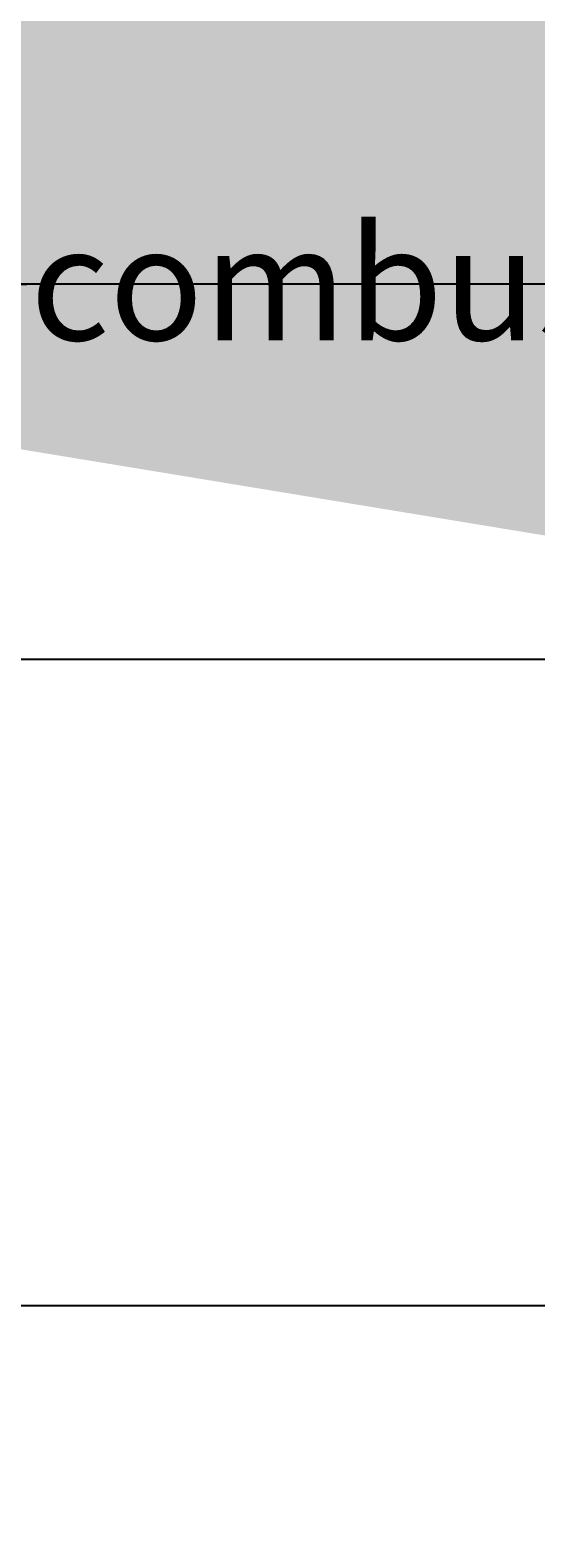
# Model space of a CAD drawing. Units: millimetres. Extents: x -22994 to 29398, y -19990 to 20176.
# Tile 53 of 135: x 216 to 229, y 25 to 65. Entities that reach past the tile are written whole.
import ezdxf
from ezdxf import colors
from ezdxf.entities.mleader import LeaderData, LeaderLine
from ezdxf.math import Vec2, Vec3

# ---------------------------------------------------------------- set-up
doc = ezdxf.new("R2010")
doc.units = ezdxf.units.MM
doc.header["$MEASUREMENT"] = 0
doc.layers.add('M-ANNO-TEXT', color=7, linetype='Continuous', lineweight=25)
doc.layers.add('M-DIMS', color=2, linetype='Continuous', lineweight=18)
doc.styles.get("Standard").update_dxf_attribs({"font": 'arial.ttf'})
doc.dimstyles.get("Standard").update_dxf_attribs({"dimtxt": 0.18, "dimasz": 10000, "dimexe": 0.18, "dimexo": 0.0625, "dimgap": 0.09, "dimtad": 0, "dimtih": 1, "dimtoh": 1, "dimdec": 0, "dimzin": 0, "dimdsep": 46, "dimtxsty": 'Standard', "dimcen": 0.09, "dimadec": 0, "dimazin": 0, "dimtfac": 1, "dimtdec": 0, "dimtofl": 0, "dimtmove": 0, "dimatfit": 3, "dimfxl": 1, "dimtolj": 1, "dimtzin": 0, "dimlwd": 30, "dimarcsym": 0})

# ---------------------------------------------------------------- blocks, each defined once
blk = doc.blocks.new('*D2')
at = {"layer": 'Defpoints', "color": 0, "transparency": 16777216}
for p in [(6.677, 10.271), (290.852, 10.271), (290.852, -5.079)]:
    blk.add_point(p, dxfattribs=at)
at = {"layer": 'M-DIMS', "color": 0, "lineweight": -2, "transparency": 16777216}
for p, q in [((6.677, 10.209), (6.677, -5.259)), ((290.852, 10.209), (290.852, -5.259))]:
    blk.add_line(p, q, dxfattribs=at)
at = {"layer": 'M-DIMS', "color": 0, "lineweight": 30, "transparency": 16777216}
for p, q in [((-9993.323, -5.079), (-19993.323, -5.079)), ((10290.852, -5.079), (20290.852, -5.079))]:
    blk.add_line(p, q, dxfattribs=at)
at = {"layer": 'M-DIMS', "color": 0, "transparency": 16777216}
for points in [[(-9993.323, 1661.588), (-9993.323, -1671.745), (6.677, -5.079)], [(10290.852, 1661.588), (10290.852, -1671.745), (290.852, -5.079)]]:
    blk.add_solid(points, dxfattribs=at)
at = {"layer": 'M-DIMS', "color": 0, "transparency": 16777216, "insert": (148.765, -5.079), "char_height": 0.18, "attachment_point": 5}
blk.add_mtext('\\A1;284.2', dxfattribs=at)
blk = doc.blocks.new('*D3')
at = {"layer": 'Defpoints', "color": 0, "transparency": 16777216}
for p in [(110.265, 204.165), (110.265, 176.366), (95.833, 127.967)]:
    blk.add_point(p, dxfattribs=at)
at = {"layer": 'M-DIMS', "color": 0, "lineweight": -2, "transparency": 16777216}
for p, q in [((95.833, 128.03), (95.833, 204.345)), ((110.265, 176.429), (110.265, 204.345))]:
    blk.add_line(p, q, dxfattribs=at)
at = {"layer": 'M-DIMS', "color": 0, "lineweight": 30, "transparency": 16777216}
for p, q in [((-9904.167, 204.165), (-19904.167, 204.165)), ((10110.265, 204.165), (20110.265, 204.165))]:
    blk.add_line(p, q, dxfattribs=at)
at = {"layer": 'M-DIMS', "color": 0, "transparency": 16777216}
for points in [[(-9904.167, 1870.832), (-9904.167, -1462.501), (95.833, 204.165)], [(10110.265, 1870.832), (10110.265, -1462.501), (110.265, 204.165)]]:
    blk.add_solid(points, dxfattribs=at)
at = {"layer": 'M-DIMS', "color": 0, "transparency": 16777216, "insert": (103.049, 204.165), "char_height": 0.18, "attachment_point": 5}
blk.add_mtext('\\A1;14.432', dxfattribs=at)
blk = doc.blocks.new('*D4')
at = {"layer": 'Defpoints', "color": 0, "transparency": 16777216}
for p in [(116.265, 204.165), (110.265, 176.366), (116.265, 176.366)]:
    blk.add_point(p, dxfattribs=at)
at = {"layer": 'M-DIMS', "color": 0, "lineweight": -2, "transparency": 16777216}
for p, q in [((110.265, 176.429), (110.265, 204.345)), ((116.265, 176.429), (116.265, 204.345))]:
    blk.add_line(p, q, dxfattribs=at)
at = {"layer": 'M-DIMS', "color": 0, "lineweight": 30, "transparency": 16777216}
for p, q in [((-9889.735, 204.165), (-19889.735, 204.165)), ((10116.265, 204.165), (20116.265, 204.165))]:
    blk.add_line(p, q, dxfattribs=at)
at = {"layer": 'M-DIMS', "color": 0, "transparency": 16777216}
for points in [[(-9889.735, 1870.832), (-9889.735, -1462.501), (110.265, 204.165)], [(10116.265, 1870.832), (10116.265, -1462.501), (116.265, 204.165)]]:
    blk.add_solid(points, dxfattribs=at)
at = {"layer": 'M-DIMS', "color": 0, "transparency": 16777216, "insert": (113.265, 204.165), "char_height": 0.18, "attachment_point": 5}
blk.add_mtext('\\A1;6', dxfattribs=at)
blk = doc.blocks.new('*D5')
at = {"layer": 'Defpoints', "color": 0, "transparency": 16777216}
for p in [(181.265, 204.165), (116.265, 176.366), (181.265, 176.366)]:
    blk.add_point(p, dxfattribs=at)
at = {"layer": 'M-DIMS', "color": 0, "lineweight": -2, "transparency": 16777216}
for p, q in [((116.265, 176.429), (116.265, 204.345)), ((181.265, 176.429), (181.265, 204.345))]:
    blk.add_line(p, q, dxfattribs=at)
at = {"layer": 'M-DIMS', "color": 0, "lineweight": 30, "transparency": 16777216}
for p, q in [((-9883.735, 204.165), (-19883.735, 204.165)), ((10181.265, 204.165), (20181.265, 204.165))]:
    blk.add_line(p, q, dxfattribs=at)
at = {"layer": 'M-DIMS', "color": 0, "transparency": 16777216}
for points in [[(-9883.735, 1870.832), (-9883.735, -1462.501), (116.265, 204.165)], [(10181.265, 1870.832), (10181.265, -1462.501), (181.265, 204.165)]]:
    blk.add_solid(points, dxfattribs=at)
at = {"layer": 'M-DIMS', "color": 0, "transparency": 16777216, "insert": (148.765, 204.165), "char_height": 0.18, "attachment_point": 5}
blk.add_mtext('\\A1;65', dxfattribs=at)
blk = doc.blocks.new('*D6')
at = {"layer": 'Defpoints', "color": 0, "transparency": 16777216}
for p in [(187.265, 204.165), (181.265, 176.366), (187.265, 176.366)]:
    blk.add_point(p, dxfattribs=at)
at = {"layer": 'M-DIMS', "color": 0, "lineweight": -2, "transparency": 16777216}
for p, q in [((181.265, 176.429), (181.265, 204.345)), ((187.265, 176.429), (187.265, 204.345))]:
    blk.add_line(p, q, dxfattribs=at)
at = {"layer": 'M-DIMS', "color": 0, "lineweight": 30, "transparency": 16777216}
for p, q in [((-9818.735, 204.165), (-19818.735, 204.165)), ((10187.265, 204.165), (20187.265, 204.165))]:
    blk.add_line(p, q, dxfattribs=at)
at = {"layer": 'M-DIMS', "color": 0, "transparency": 16777216}
for points in [[(-9818.735, 1870.832), (-9818.735, -1462.501), (181.265, 204.165)], [(10187.265, 1870.832), (10187.265, -1462.501), (187.265, 204.165)]]:
    blk.add_solid(points, dxfattribs=at)
at = {"layer": 'M-DIMS', "color": 0, "transparency": 16777216, "insert": (184.265, 204.165), "char_height": 0.18, "attachment_point": 5}
blk.add_mtext('\\A1;6', dxfattribs=at)
blk = doc.blocks.new('*D7')
at = {"layer": 'Defpoints', "color": 0, "transparency": 16777216}
for p in [(201.697, 204.165), (187.265, 176.366), (201.697, 127.967)]:
    blk.add_point(p, dxfattribs=at)
at = {"layer": 'M-DIMS', "color": 0, "lineweight": -2, "transparency": 16777216}
for p, q in [((187.265, 176.429), (187.265, 204.345)), ((201.697, 128.03), (201.697, 204.345))]:
    blk.add_line(p, q, dxfattribs=at)
at = {"layer": 'M-DIMS', "color": 0, "lineweight": 30, "transparency": 16777216}
for p, q in [((-9812.735, 204.165), (-19812.735, 204.165)), ((10201.697, 204.165), (20201.697, 204.165))]:
    blk.add_line(p, q, dxfattribs=at)
at = {"layer": 'M-DIMS', "color": 0, "transparency": 16777216}
for points in [[(-9812.735, 1870.832), (-9812.735, -1462.501), (187.265, 204.165)], [(10201.697, 1870.832), (10201.697, -1462.501), (201.697, 204.165)]]:
    blk.add_solid(points, dxfattribs=at)
at = {"layer": 'M-DIMS', "color": 0, "transparency": 16777216, "insert": (194.481, 204.165), "char_height": 0.18, "attachment_point": 5}
blk.add_mtext('\\A1;14.432', dxfattribs=at)
blk = doc.blocks.new('*D8')
at = {"layer": 'Defpoints', "color": 0, "transparency": 16777216}
for p in [(227.648, 204.165), (227.648, 146.73), (201.697, 127.967)]:
    blk.add_point(p, dxfattribs=at)
at = {"layer": 'M-DIMS', "color": 0, "lineweight": -2, "transparency": 16777216}
for p, q in [((201.697, 128.03), (201.697, 204.345)), ((227.648, 146.792), (227.648, 204.345))]:
    blk.add_line(p, q, dxfattribs=at)
at = {"layer": 'M-DIMS', "color": 0, "lineweight": 30, "transparency": 16777216}
for p, q in [((-9798.303, 204.165), (-19798.303, 204.165)), ((10227.648, 204.165), (20227.648, 204.165))]:
    blk.add_line(p, q, dxfattribs=at)
at = {"layer": 'M-DIMS', "color": 0, "transparency": 16777216}
for points in [[(-9798.303, 1870.832), (-9798.303, -1462.501), (201.697, 204.165)], [(10227.648, 1870.832), (10227.648, -1462.501), (227.648, 204.165)]]:
    blk.add_solid(points, dxfattribs=at)
at = {"layer": 'M-DIMS', "color": 0, "transparency": 16777216, "insert": (214.673, 204.165), "char_height": 0.18, "attachment_point": 5}
blk.add_mtext('\\A1;25.95', dxfattribs=at)
blk = doc.blocks.new('*D9')
at = {"layer": 'Defpoints', "color": 0, "transparency": 16777216}
for p in [(187.265, 176.366), (306.202, 176.366), (290.852, 10.271)]:
    blk.add_point(p, dxfattribs=at)
at = {"layer": 'M-DIMS', "color": 0, "lineweight": 30, "transparency": 16777216}
for p, q in [((306.202, 10176.366), (306.202, 20176.366)), ((306.202, -9989.729), (306.202, -19989.729))]:
    blk.add_line(p, q, dxfattribs=at)
at = {"layer": 'M-DIMS', "color": 0, "lineweight": -2, "transparency": 16777216}
for p, q in [((187.327, 176.366), (306.382, 176.366)), ((290.915, 10.271), (306.382, 10.271))]:
    blk.add_line(p, q, dxfattribs=at)
at = {"layer": 'M-DIMS', "color": 0, "transparency": 16777216}
for points in [[(-1360.465, 10176.366), (1972.869, 10176.366), (306.202, 176.366)], [(-1360.465, -9989.729), (1972.869, -9989.729), (306.202, 10.271)]]:
    blk.add_solid(points, dxfattribs=at)
at = {"layer": 'M-DIMS', "color": 0, "transparency": 16777216, "insert": (306.202, 93.319), "char_height": 0.18, "attachment_point": 5}
blk.add_mtext('\\A1;166.1', dxfattribs=at)
blk = doc.blocks.new('*D10')
at = {"layer": 'Defpoints', "color": 0, "transparency": 16777216}
for p in [(125.65, 136.071), (133.346, 136.071), (133.346, -5.079)]:
    blk.add_point(p, dxfattribs=at)
at = {"layer": 'M-DIMS', "color": 0, "lineweight": -2, "transparency": 16777216}
for p, q in [((125.65, 136.009), (125.65, -5.259)), ((133.346, 136.009), (133.346, -5.259))]:
    blk.add_line(p, q, dxfattribs=at)
at = {"layer": 'M-DIMS', "color": 0, "lineweight": 30, "transparency": 16777216}
for p, q in [((-9874.35, -5.079), (-19874.35, -5.079)), ((10133.346, -5.079), (20133.346, -5.079))]:
    blk.add_line(p, q, dxfattribs=at)
at = {"layer": 'M-DIMS', "color": 0, "transparency": 16777216}
for points in [[(-9874.35, 1661.588), (-9874.35, -1671.745), (125.65, -5.079)], [(10133.346, 1661.588), (10133.346, -1671.745), (133.346, -5.079)]]:
    blk.add_solid(points, dxfattribs=at)
at = {"layer": 'M-DIMS', "color": 0, "transparency": 16777216, "insert": (129.498, -5.079), "char_height": 0.18, "attachment_point": 5}
blk.add_mtext('\\A1;7.696', dxfattribs=at)
blk = doc.blocks.new('*D11')
at = {"layer": 'Defpoints', "color": 0, "transparency": 16777216}
for p in [(133.346, 136.071), (135.65, 136.071), (135.65, -5.079)]:
    blk.add_point(p, dxfattribs=at)
at = {"layer": 'M-DIMS', "color": 0, "lineweight": -2, "transparency": 16777216}
for p, q in [((133.346, 136.009), (133.346, -5.259)), ((135.65, 136.009), (135.65, -5.259))]:
    blk.add_line(p, q, dxfattribs=at)
at = {"layer": 'M-DIMS', "color": 0, "lineweight": 30, "transparency": 16777216}
for p, q in [((-9866.654, -5.079), (-19866.654, -5.079)), ((10135.65, -5.079), (20135.65, -5.079))]:
    blk.add_line(p, q, dxfattribs=at)
at = {"layer": 'M-DIMS', "color": 0, "transparency": 16777216}
for points in [[(-9866.654, 1661.588), (-9866.654, -1671.745), (133.346, -5.079)], [(10135.65, 1661.588), (10135.65, -1671.745), (135.65, -5.079)]]:
    blk.add_solid(points, dxfattribs=at)
at = {"layer": 'M-DIMS', "color": 0, "transparency": 16777216, "insert": (134.498, -5.079), "char_height": 0.18, "attachment_point": 5}
blk.add_mtext('\\A1;2.304', dxfattribs=at)
blk = doc.blocks.new('*D12')
at = {"layer": 'Defpoints', "color": 0, "transparency": 16777216}
for p in [(135.65, 136.071), (145.65, 136.071), (145.65, -5.079)]:
    blk.add_point(p, dxfattribs=at)
at = {"layer": 'M-DIMS', "color": 0, "lineweight": -2, "transparency": 16777216}
for p, q in [((135.65, 136.009), (135.65, -5.259)), ((145.65, 136.009), (145.65, -5.259))]:
    blk.add_line(p, q, dxfattribs=at)
at = {"layer": 'M-DIMS', "color": 0, "lineweight": 30, "transparency": 16777216}
for p, q in [((-9864.35, -5.079), (-19864.35, -5.079)), ((10145.65, -5.079), (20145.65, -5.079))]:
    blk.add_line(p, q, dxfattribs=at)
at = {"layer": 'M-DIMS', "color": 0, "transparency": 16777216}
for points in [[(-9864.35, 1661.588), (-9864.35, -1671.745), (135.65, -5.079)], [(10145.65, 1661.588), (10145.65, -1671.745), (145.65, -5.079)]]:
    blk.add_solid(points, dxfattribs=at)
at = {"layer": 'M-DIMS', "color": 0, "transparency": 16777216, "insert": (140.65, -5.079), "char_height": 0.18, "attachment_point": 5}
blk.add_mtext('\\A1;10', dxfattribs=at)
blk = doc.blocks.new('*D13')
at = {"layer": 'Defpoints', "color": 0, "transparency": 16777216}
for p in [(145.65, 136.071), (155.65, 136.071), (155.65, -5.079)]:
    blk.add_point(p, dxfattribs=at)
at = {"layer": 'M-DIMS', "color": 0, "lineweight": -2, "transparency": 16777216}
for p, q in [((145.65, 136.009), (145.65, -5.259)), ((155.65, 136.009), (155.65, -5.259))]:
    blk.add_line(p, q, dxfattribs=at)
at = {"layer": 'M-DIMS', "color": 0, "lineweight": 30, "transparency": 16777216}
for p, q in [((-9854.35, -5.079), (-19854.35, -5.079)), ((10155.65, -5.079), (20155.65, -5.079))]:
    blk.add_line(p, q, dxfattribs=at)
at = {"layer": 'M-DIMS', "color": 0, "transparency": 16777216}
for points in [[(-9854.35, 1661.588), (-9854.35, -1671.745), (145.65, -5.079)], [(10155.65, 1661.588), (10155.65, -1671.745), (155.65, -5.079)]]:
    blk.add_solid(points, dxfattribs=at)
at = {"layer": 'M-DIMS', "color": 0, "transparency": 16777216, "insert": (150.65, -5.079), "char_height": 0.18, "attachment_point": 5}
blk.add_mtext('\\A1;10', dxfattribs=at)
blk = doc.blocks.new('*D14')
at = {"layer": 'Defpoints', "color": 0, "transparency": 16777216}
for p in [(155.65, 136.071), (165.65, 136.071), (165.65, -5.079)]:
    blk.add_point(p, dxfattribs=at)
at = {"layer": 'M-DIMS', "color": 0, "lineweight": -2, "transparency": 16777216}
for p, q in [((155.65, 136.009), (155.65, -5.259)), ((165.65, 136.009), (165.65, -5.259))]:
    blk.add_line(p, q, dxfattribs=at)
at = {"layer": 'M-DIMS', "color": 0, "lineweight": 30, "transparency": 16777216}
for p, q in [((-9844.35, -5.079), (-19844.35, -5.079)), ((10165.65, -5.079), (20165.65, -5.079))]:
    blk.add_line(p, q, dxfattribs=at)
at = {"layer": 'M-DIMS', "color": 0, "transparency": 16777216}
for points in [[(-9844.35, 1661.588), (-9844.35, -1671.745), (155.65, -5.079)], [(10165.65, 1661.588), (10165.65, -1671.745), (165.65, -5.079)]]:
    blk.add_solid(points, dxfattribs=at)
at = {"layer": 'M-DIMS', "color": 0, "transparency": 16777216, "insert": (160.65, -5.079), "char_height": 0.18, "attachment_point": 5}
blk.add_mtext('\\A1;10', dxfattribs=at)
blk = doc.blocks.new('*D15')
at = {"layer": 'Defpoints', "color": 0, "transparency": 16777216}
for p in [(173.346, 154.788), (173.346, 136.071), (306.202, 136.071)]:
    blk.add_point(p, dxfattribs=at)
at = {"layer": 'M-DIMS', "color": 0, "lineweight": 30, "transparency": 16777216}
for p, q in [((306.202, 10154.788), (306.202, 20154.788)), ((306.202, -9863.929), (306.202, -19863.929))]:
    blk.add_line(p, q, dxfattribs=at)
at = {"layer": 'M-DIMS', "color": 0, "lineweight": -2, "transparency": 16777216}
for p, q in [((173.408, 154.788), (306.382, 154.788)), ((173.408, 136.071), (306.382, 136.071))]:
    blk.add_line(p, q, dxfattribs=at)
at = {"layer": 'M-DIMS', "color": 0, "transparency": 16777216}
for points in [[(-1360.465, 10154.788), (1972.869, 10154.788), (306.202, 154.788)], [(-1360.465, -9863.929), (1972.869, -9863.929), (306.202, 136.071)]]:
    blk.add_solid(points, dxfattribs=at)
at = {"layer": 'M-DIMS', "color": 0, "transparency": 16777216, "insert": (306.202, 145.43), "char_height": 0.18, "attachment_point": 5}
blk.add_mtext('\\A1;18.717', dxfattribs=at)
blk = doc.blocks.new('*D16')
at = {"layer": 'Defpoints', "color": 0, "transparency": 16777216}
for p in [(120.17, 204.165), (110.466, 48.035), (120.17, 48.035)]:
    blk.add_point(p, dxfattribs=at)
at = {"layer": 'M-DIMS', "color": 0, "lineweight": -2, "transparency": 16777216}
for p, q in [((110.466, 48.097), (110.466, 204.345)), ((120.17, 48.097), (120.17, 204.345))]:
    blk.add_line(p, q, dxfattribs=at)
at = {"layer": 'M-DIMS', "color": 0, "lineweight": 30, "transparency": 16777216}
for p, q in [((-9889.534, 204.165), (-19889.534, 204.165)), ((10120.17, 204.165), (20120.17, 204.165))]:
    blk.add_line(p, q, dxfattribs=at)
at = {"layer": 'M-DIMS', "color": 0, "transparency": 16777216}
for points in [[(-9889.534, 1870.832), (-9889.534, -1462.501), (110.466, 204.165)], [(10120.17, 1870.832), (10120.17, -1462.501), (120.17, 204.165)]]:
    blk.add_solid(points, dxfattribs=at)
at = {"layer": 'M-DIMS', "color": 0, "transparency": 16777216, "insert": (115.318, 204.165), "char_height": 0.18, "attachment_point": 5}
blk.add_mtext('\\A1;9.704', dxfattribs=at)
blk = doc.blocks.new('*D17')
at = {"layer": 'Defpoints', "color": 0, "transparency": 16777216}
for p in [(126.17, 204.165), (120.17, 48.035), (126.17, 48.035)]:
    blk.add_point(p, dxfattribs=at)
at = {"layer": 'M-DIMS', "color": 0, "lineweight": -2, "transparency": 16777216}
for p, q in [((120.17, 48.097), (120.17, 204.345)), ((126.17, 48.097), (126.17, 204.345))]:
    blk.add_line(p, q, dxfattribs=at)
at = {"layer": 'M-DIMS', "color": 0, "lineweight": 30, "transparency": 16777216}
for p, q in [((-9879.83, 204.165), (-19879.83, 204.165)), ((10126.17, 204.165), (20126.17, 204.165))]:
    blk.add_line(p, q, dxfattribs=at)
at = {"layer": 'M-DIMS', "color": 0, "transparency": 16777216}
for points in [[(-9879.83, 1870.832), (-9879.83, -1462.501), (120.17, 204.165)], [(10126.17, 1870.832), (10126.17, -1462.501), (126.17, 204.165)]]:
    blk.add_solid(points, dxfattribs=at)
at = {"layer": 'M-DIMS', "color": 0, "transparency": 16777216, "insert": (123.17, 204.165), "char_height": 0.18, "attachment_point": 5}
blk.add_mtext('\\A1;6', dxfattribs=at)
blk = doc.blocks.new('*D18')
at = {"layer": 'Defpoints', "color": 0, "transparency": 16777216}
for p in [(132.17, 204.165), (126.17, 48.035), (132.17, 48.035)]:
    blk.add_point(p, dxfattribs=at)
at = {"layer": 'M-DIMS', "color": 0, "lineweight": -2, "transparency": 16777216}
for p, q in [((126.17, 48.097), (126.17, 204.345)), ((132.17, 48.097), (132.17, 204.345))]:
    blk.add_line(p, q, dxfattribs=at)
at = {"layer": 'M-DIMS', "color": 0, "lineweight": 30, "transparency": 16777216}
for p, q in [((-9873.83, 204.165), (-19873.83, 204.165)), ((10132.17, 204.165), (20132.17, 204.165))]:
    blk.add_line(p, q, dxfattribs=at)
at = {"layer": 'M-DIMS', "color": 0, "transparency": 16777216}
for points in [[(-9873.83, 1870.832), (-9873.83, -1462.501), (126.17, 204.165)], [(10132.17, 1870.832), (10132.17, -1462.501), (132.17, 204.165)]]:
    blk.add_solid(points, dxfattribs=at)
at = {"layer": 'M-DIMS', "color": 0, "transparency": 16777216, "insert": (129.17, 204.165), "char_height": 0.18, "attachment_point": 5}
blk.add_mtext('\\A1;6', dxfattribs=at)
blk = doc.blocks.new('*D19')
at = {"layer": 'Defpoints', "color": 0, "transparency": 16777216}
for p in [(138.17, 204.165), (132.17, 48.035), (138.17, 48.035)]:
    blk.add_point(p, dxfattribs=at)
at = {"layer": 'M-DIMS', "color": 0, "lineweight": -2, "transparency": 16777216}
for p, q in [((132.17, 48.097), (132.17, 204.345)), ((138.17, 48.097), (138.17, 204.345))]:
    blk.add_line(p, q, dxfattribs=at)
at = {"layer": 'M-DIMS', "color": 0, "lineweight": 30, "transparency": 16777216}
for p, q in [((-9867.83, 204.165), (-19867.83, 204.165)), ((10138.17, 204.165), (20138.17, 204.165))]:
    blk.add_line(p, q, dxfattribs=at)
at = {"layer": 'M-DIMS', "color": 0, "transparency": 16777216}
for points in [[(-9867.83, 1870.832), (-9867.83, -1462.501), (132.17, 204.165)], [(10138.17, 1870.832), (10138.17, -1462.501), (138.17, 204.165)]]:
    blk.add_solid(points, dxfattribs=at)
at = {"layer": 'M-DIMS', "color": 0, "transparency": 16777216, "insert": (135.17, 204.165), "char_height": 0.18, "attachment_point": 5}
blk.add_mtext('\\A1;6', dxfattribs=at)
blk = doc.blocks.new('*D20')
at = {"layer": 'Defpoints', "color": 0, "transparency": 16777216}
for p in [(144.17, 204.165), (138.17, 48.035), (144.17, 48.035)]:
    blk.add_point(p, dxfattribs=at)
at = {"layer": 'M-DIMS', "color": 0, "lineweight": -2, "transparency": 16777216}
for p, q in [((138.17, 48.097), (138.17, 204.345)), ((144.17, 48.097), (144.17, 204.345))]:
    blk.add_line(p, q, dxfattribs=at)
at = {"layer": 'M-DIMS', "color": 0, "lineweight": 30, "transparency": 16777216}
for p, q in [((-9861.83, 204.165), (-19861.83, 204.165)), ((10144.17, 204.165), (20144.17, 204.165))]:
    blk.add_line(p, q, dxfattribs=at)
at = {"layer": 'M-DIMS', "color": 0, "transparency": 16777216}
for points in [[(-9861.83, 1870.832), (-9861.83, -1462.501), (138.17, 204.165)], [(10144.17, 1870.832), (10144.17, -1462.501), (144.17, 204.165)]]:
    blk.add_solid(points, dxfattribs=at)
at = {"layer": 'M-DIMS', "color": 0, "transparency": 16777216, "insert": (141.17, 204.165), "char_height": 0.18, "attachment_point": 5}
blk.add_mtext('\\A1;6', dxfattribs=at)
blk = doc.blocks.new('*D21')
at = {"layer": 'Defpoints', "color": 0, "transparency": 16777216}
for p in [(149.116, 204.165), (144.17, 48.035), (149.116, 48.035)]:
    blk.add_point(p, dxfattribs=at)
at = {"layer": 'M-DIMS', "color": 0, "lineweight": -2, "transparency": 16777216}
for p, q in [((144.17, 48.097), (144.17, 204.345)), ((149.116, 48.097), (149.116, 204.345))]:
    blk.add_line(p, q, dxfattribs=at)
at = {"layer": 'M-DIMS', "color": 0, "lineweight": 30, "transparency": 16777216}
for p, q in [((-9855.83, 204.165), (-19855.83, 204.165)), ((10149.116, 204.165), (20149.116, 204.165))]:
    blk.add_line(p, q, dxfattribs=at)
at = {"layer": 'M-DIMS', "color": 0, "transparency": 16777216}
for points in [[(-9855.83, 1870.832), (-9855.83, -1462.501), (144.17, 204.165)], [(10149.116, 1870.832), (10149.116, -1462.501), (149.116, 204.165)]]:
    blk.add_solid(points, dxfattribs=at)
at = {"layer": 'M-DIMS', "color": 0, "transparency": 16777216, "insert": (146.643, 204.165), "char_height": 0.18, "attachment_point": 5}
blk.add_mtext('\\A1;4.945', dxfattribs=at)
blk = doc.blocks.new('*D22')
at = {"layer": 'Defpoints', "color": 0, "transparency": 16777216}
for p in [(149.116, 30.99), (155.116, 30.99), (155.116, -5.079)]:
    blk.add_point(p, dxfattribs=at)
at = {"layer": 'M-DIMS', "color": 0, "lineweight": -2, "transparency": 16777216}
for p, q in [((149.116, 30.927), (149.116, -5.259)), ((155.116, 30.927), (155.116, -5.259))]:
    blk.add_line(p, q, dxfattribs=at)
at = {"layer": 'M-DIMS', "color": 0, "lineweight": 30, "transparency": 16777216}
for p, q in [((-9850.884, -5.079), (-19850.884, -5.079)), ((10155.116, -5.079), (20155.116, -5.079))]:
    blk.add_line(p, q, dxfattribs=at)
at = {"layer": 'M-DIMS', "color": 0, "transparency": 16777216}
for points in [[(-9850.884, 1661.588), (-9850.884, -1671.745), (149.116, -5.079)], [(10155.116, 1661.588), (10155.116, -1671.745), (155.116, -5.079)]]:
    blk.add_solid(points, dxfattribs=at)
at = {"layer": 'M-DIMS', "color": 0, "transparency": 16777216, "insert": (152.116, -5.079), "char_height": 0.18, "attachment_point": 5}
blk.add_mtext('\\A1;6', dxfattribs=at)
blk = doc.blocks.new('*D23')
at = {"layer": 'Defpoints', "color": 0, "transparency": 16777216}
for p in [(155.116, 30.99), (161.116, 30.99), (161.116, -5.079)]:
    blk.add_point(p, dxfattribs=at)
at = {"layer": 'M-DIMS', "color": 0, "lineweight": -2, "transparency": 16777216}
for p, q in [((155.116, 30.927), (155.116, -5.259)), ((161.116, 30.927), (161.116, -5.259))]:
    blk.add_line(p, q, dxfattribs=at)
at = {"layer": 'M-DIMS', "color": 0, "lineweight": 30, "transparency": 16777216}
for p, q in [((-9844.884, -5.079), (-19844.884, -5.079)), ((10161.116, -5.079), (20161.116, -5.079))]:
    blk.add_line(p, q, dxfattribs=at)
at = {"layer": 'M-DIMS', "color": 0, "transparency": 16777216}
for points in [[(-9844.884, 1661.588), (-9844.884, -1671.745), (155.116, -5.079)], [(10161.116, 1661.588), (10161.116, -1671.745), (161.116, -5.079)]]:
    blk.add_solid(points, dxfattribs=at)
at = {"layer": 'M-DIMS', "color": 0, "transparency": 16777216, "insert": (158.116, -5.079), "char_height": 0.18, "attachment_point": 5}
blk.add_mtext('\\A1;6', dxfattribs=at)
blk = doc.blocks.new('*D24')
at = {"layer": 'Defpoints', "color": 0, "transparency": 16777216}
for p in [(161.116, 30.99), (166.439, 30.99), (166.439, -5.079)]:
    blk.add_point(p, dxfattribs=at)
at = {"layer": 'M-DIMS', "color": 0, "lineweight": -2, "transparency": 16777216}
for p, q in [((161.116, 30.927), (161.116, -5.259)), ((166.439, 30.927), (166.439, -5.259))]:
    blk.add_line(p, q, dxfattribs=at)
at = {"layer": 'M-DIMS', "color": 0, "lineweight": 30, "transparency": 16777216}
for p, q in [((-9838.884, -5.079), (-19838.884, -5.079)), ((10166.439, -5.079), (20166.439, -5.079))]:
    blk.add_line(p, q, dxfattribs=at)
at = {"layer": 'M-DIMS', "color": 0, "transparency": 16777216}
for points in [[(-9838.884, 1661.588), (-9838.884, -1671.745), (161.116, -5.079)], [(10166.439, 1661.588), (10166.439, -1671.745), (166.439, -5.079)]]:
    blk.add_solid(points, dxfattribs=at)
at = {"layer": 'M-DIMS', "color": 0, "transparency": 16777216, "insert": (163.777, -5.079), "char_height": 0.18, "attachment_point": 5}
blk.add_mtext('\\A1;5.323', dxfattribs=at)
blk = doc.blocks.new('*D25')
at = {"layer": 'Defpoints', "color": 0, "transparency": 16777216}
for p in [(166.439, 30.99), (172.439, 30.99), (172.439, -5.079)]:
    blk.add_point(p, dxfattribs=at)
at = {"layer": 'M-DIMS', "color": 0, "lineweight": -2, "transparency": 16777216}
for p, q in [((166.439, 30.927), (166.439, -5.259)), ((172.439, 30.927), (172.439, -5.259))]:
    blk.add_line(p, q, dxfattribs=at)
at = {"layer": 'M-DIMS', "color": 0, "lineweight": 30, "transparency": 16777216}
for p, q in [((-9833.561, -5.079), (-19833.561, -5.079)), ((10172.439, -5.079), (20172.439, -5.079))]:
    blk.add_line(p, q, dxfattribs=at)
at = {"layer": 'M-DIMS', "color": 0, "transparency": 16777216}
for points in [[(-9833.561, 1661.588), (-9833.561, -1671.745), (166.439, -5.079)], [(10172.439, 1661.588), (10172.439, -1671.745), (172.439, -5.079)]]:
    blk.add_solid(points, dxfattribs=at)
at = {"layer": 'M-DIMS', "color": 0, "transparency": 16777216, "insert": (169.439, -5.079), "char_height": 0.18, "attachment_point": 5}
blk.add_mtext('\\A1;6', dxfattribs=at)
blk = doc.blocks.new('*D26')
at = {"layer": 'Defpoints', "color": 0, "transparency": 16777216}
for p in [(172.439, 30.99), (178.439, 30.99), (178.439, -5.079)]:
    blk.add_point(p, dxfattribs=at)
at = {"layer": 'M-DIMS', "color": 0, "lineweight": -2, "transparency": 16777216}
for p, q in [((172.439, 30.927), (172.439, -5.259)), ((178.439, 30.927), (178.439, -5.259))]:
    blk.add_line(p, q, dxfattribs=at)
at = {"layer": 'M-DIMS', "color": 0, "lineweight": 30, "transparency": 16777216}
for p, q in [((-9827.561, -5.079), (-19827.561, -5.079)), ((10178.439, -5.079), (20178.439, -5.079))]:
    blk.add_line(p, q, dxfattribs=at)
at = {"layer": 'M-DIMS', "color": 0, "transparency": 16777216}
for points in [[(-9827.561, 1661.588), (-9827.561, -1671.745), (172.439, -5.079)], [(10178.439, 1661.588), (10178.439, -1671.745), (178.439, -5.079)]]:
    blk.add_solid(points, dxfattribs=at)
at = {"layer": 'M-DIMS', "color": 0, "transparency": 16777216, "insert": (175.439, -5.079), "char_height": 0.18, "attachment_point": 5}
blk.add_mtext('\\A1;6', dxfattribs=at)
blk = doc.blocks.new('*D27')
at = {"layer": 'Defpoints', "color": 0, "transparency": 16777216}
for p in [(178.439, 30.99), (188.117, 30.99), (188.117, -5.079)]:
    blk.add_point(p, dxfattribs=at)
at = {"layer": 'M-DIMS', "color": 0, "lineweight": -2, "transparency": 16777216}
for p, q in [((178.439, 30.927), (178.439, -5.259)), ((188.117, 30.927), (188.117, -5.259))]:
    blk.add_line(p, q, dxfattribs=at)
at = {"layer": 'M-DIMS', "color": 0, "lineweight": 30, "transparency": 16777216}
for p, q in [((-9821.561, -5.079), (-19821.561, -5.079)), ((10188.117, -5.079), (20188.117, -5.079))]:
    blk.add_line(p, q, dxfattribs=at)
at = {"layer": 'M-DIMS', "color": 0, "transparency": 16777216}
for points in [[(-9821.561, 1661.588), (-9821.561, -1671.745), (178.439, -5.079)], [(10188.117, 1661.588), (10188.117, -1671.745), (188.117, -5.079)]]:
    blk.add_solid(points, dxfattribs=at)
at = {"layer": 'M-DIMS', "color": 0, "transparency": 16777216, "insert": (183.278, -5.079), "char_height": 0.18, "attachment_point": 5}
blk.add_mtext('\\A1;9.679', dxfattribs=at)
blk = doc.blocks.new('*D28')
at = {"layer": 'Defpoints', "color": 0, "transparency": 16777216}
for p in [(188.117, 48.035), (306.202, 48.035), (188.117, 30.99)]:
    blk.add_point(p, dxfattribs=at)
at = {"layer": 'M-DIMS', "color": 0, "lineweight": 30, "transparency": 16777216}
for p, q in [((306.202, 10048.035), (306.202, 20048.035)), ((306.202, -9969.01), (306.202, -19969.01))]:
    blk.add_line(p, q, dxfattribs=at)
at = {"layer": 'M-DIMS', "color": 0, "lineweight": -2, "transparency": 16777216}
for p, q in [((188.18, 48.035), (306.382, 48.035)), ((188.18, 30.99), (306.382, 30.99))]:
    blk.add_line(p, q, dxfattribs=at)
at = {"layer": 'M-DIMS', "color": 0, "transparency": 16777216}
for points in [[(-1360.465, 10048.035), (1972.869, 10048.035), (306.202, 48.035)], [(-1360.465, -9969.01), (1972.869, -9969.01), (306.202, 30.99)]]:
    blk.add_solid(points, dxfattribs=at)
at = {"layer": 'M-DIMS', "color": 0, "transparency": 16777216, "insert": (306.202, 39.512), "char_height": 0.18, "attachment_point": 5}
blk.add_mtext('\\A1;17.045', dxfattribs=at)
blk = doc.blocks.new('*D29')
at = {"layer": 'Defpoints', "color": 0, "transparency": 16777216}
for p in [(36.801, 80.045), (64.03, 80.045)]:
    blk.add_point(p, dxfattribs=at)
at = {"layer": 'M-DIMS', "color": 0, "lineweight": -2, "transparency": 16777216}
for p, q in [((50.325, 80.045), (50.505, 80.045)), ((50.415, 79.955), (50.415, 80.135))]:
    blk.add_line(p, q, dxfattribs=at)
at = {"layer": 'M-DIMS', "color": 0, "lineweight": 30, "transparency": 16777216}
blk.add_line((20064.03, 80.03), (10064.03, 80.038), dxfattribs=at)
at = {"layer": 'M-DIMS', "color": 0, "transparency": 16777216}
blk.add_solid([(10064.031, 1746.704), (10064.028, -1586.629), (64.03, 80.045)], dxfattribs=at)
at = {"layer": 'M-DIMS', "color": 0, "transparency": 16777216, "insert": (20064.521, 80.03), "char_height": 0.18, "attachment_point": 5}
blk.add_mtext('\\A1;∅27.23', dxfattribs=at)
blk = doc.blocks.new('*D30')
at = {"layer": 'Defpoints', "color": 0, "transparency": 16777216}
for p in [(216.315, 146.729), (238.982, 146.73)]:
    blk.add_point(p, dxfattribs=at)
at = {"layer": 'M-DIMS', "color": 0, "lineweight": 30, "transparency": 16777216}
blk.add_line((20238.982, 147.496), (10238.982, 147.113), dxfattribs=at)
at = {"layer": 'M-DIMS', "color": 0, "lineweight": -2, "transparency": 16777216}
for p, q in [((227.558, 146.73), (227.738, 146.73)), ((227.648, 146.64), (227.648, 146.82))]:
    blk.add_line(p, q, dxfattribs=at)
at = {"layer": 'M-DIMS', "color": 0, "transparency": 16777216}
blk.add_solid([(10238.918, 1813.78), (10239.046, -1519.554), (238.982, 146.73)], dxfattribs=at)
at = {"layer": 'M-DIMS', "color": 0, "transparency": 16777216, "insert": (20239.544, 147.496), "char_height": 0.18, "attachment_point": 5}
blk.add_mtext('\\A1;∅22.667', dxfattribs=at)
blk = doc.blocks.new('*D31')
at = {"layer": 'Defpoints', "color": 0, "transparency": 16777216}
for p in [(223.164, 146.729), (232.133, 146.73)]:
    blk.add_point(p, dxfattribs=at)
at = {"layer": 'M-DIMS', "color": 0, "lineweight": 30, "transparency": 16777216}
blk.add_line((20232.133, 148.666), (10232.133, 147.698), dxfattribs=at)
at = {"layer": 'M-DIMS', "color": 0, "lineweight": -2, "transparency": 16777216}
for p, q in [((227.558, 146.73), (227.738, 146.73)), ((227.648, 146.64), (227.648, 146.82))]:
    blk.add_line(p, q, dxfattribs=at)
at = {"layer": 'M-DIMS', "color": 0, "transparency": 16777216}
blk.add_solid([(10231.971, 1814.364), (10232.294, -1518.969), (232.133, 146.73)], dxfattribs=at)
at = {"layer": 'M-DIMS', "color": 0, "transparency": 16777216, "insert": (20232.625, 148.666), "char_height": 0.18, "attachment_point": 5}
blk.add_mtext('\\A1;∅8.969', dxfattribs=at)
blk = doc.blocks.new('*D36')
at = {"layer": 'Defpoints', "color": 0, "transparency": 16777216}
for p in [(46.39, 31.303), (46.387, 26.593)]:
    blk.add_point(p, dxfattribs=at)
at = {"layer": 'M-DIMS', "color": 0, "lineweight": 30, "transparency": 16777216}
for p, q in [((57.15, 20031.301), (51.77, 10031.302)), ((10057.15, 20031.301), (57.15, 20031.301))]:
    blk.add_line(p, q, dxfattribs=at)
at = {"layer": 'M-DIMS', "color": 0, "lineweight": -2, "transparency": 16777216}
for p, q in [((46.389, 28.858), (46.389, 29.038)), ((46.299, 28.948), (46.479, 28.948))]:
    blk.add_line(p, q, dxfattribs=at)
at = {"layer": 'M-DIMS', "color": 0, "transparency": 16777216}
blk.add_solid([(-1614.896, 10032.199), (1718.436, 10030.405), (46.39, 31.303)], dxfattribs=at)
at = {"layer": 'M-DIMS', "color": 0, "transparency": 16777216, "insert": (10057.554, 20031.301), "char_height": 0.18, "attachment_point": 5}
blk.add_mtext('\\A1;∅4.71', dxfattribs=at)
blk = doc.blocks.new('*D37')
at = {"layer": 'Defpoints', "color": 0, "transparency": 16777216}
for p in [(54.834, 118.615), (59.494, 118.614)]:
    blk.add_point(p, dxfattribs=at)
at = {"layer": 'M-DIMS', "color": 0, "lineweight": -2, "transparency": 16777216}
for p, q in [((57.074, 118.614), (57.254, 118.614)), ((57.164, 118.524), (57.164, 118.704))]:
    blk.add_line(p, q, dxfattribs=at)
at = {"layer": 'M-DIMS', "color": 0, "lineweight": 30, "transparency": 16777216}
blk.add_line((20059.493, 116.253), (10059.494, 117.434), dxfattribs=at)
at = {"layer": 'M-DIMS', "color": 0, "transparency": 16777216}
blk.add_solid([(10059.69, 1784.1), (10059.297, -1549.233), (59.494, 118.614)], dxfattribs=at)
at = {"layer": 'M-DIMS', "color": 0, "transparency": 16777216, "insert": (20059.985, 116.253), "char_height": 0.18, "attachment_point": 5}
blk.add_mtext('\\A1;∅4.659', dxfattribs=at)

msp = doc.modelspace()

# ---------------------------------------------------------------- dimensions: what is measured, and where the dimension line sits
at = {"layer": 'M-DIMS'}
for base, p1, p2, override, picture, middle in [((306.202, 176.3662), (290.852, 10.2713), (187.2647, 176.3662), {"dimdec": 1, "dimlfac": 1, "dimrnd": 0, "dimzin": 0, "dimdsep": 46, "dimlunit": 2}, '*D9', (306.202, 93.3187)), ((306.202, 136.0713), (173.3459, 154.788), (173.3459, 136.0713), {"dimdec": 3, "dimlfac": 1, "dimrnd": 0, "dimzin": 0, "dimdsep": 46, "dimlunit": 2}, '*D15', (306.202, 145.4297)), ((306.202, 48.0349), (188.1175, 30.9895), (188.1175, 48.0349), {"dimdec": 3, "dimlfac": 1, "dimrnd": 0, "dimzin": 0, "dimdsep": 46, "dimlunit": 2}, '*D28', (306.202, 39.5122))]:
    dim = msp.add_linear_dim(base=base, p1=p1, p2=p2, angle=90, dimstyle='Standard', override=override, dxfattribs=at)
    dim.commit()
    dim.dimension.update_dxf_attribs({"geometry": picture, "text_midpoint": middle})
for p1, p2, override, picture, middle in [((46.3875, 26.5934), (46.39, 31.3035), {"dimdec": 2, "dimlfac": 1, "dimrnd": 0, "dimzin": 0, "dimdsep": 46, "dimlunit": 2}, '*D36', (10057.5542, 20031.3006)), ((223.1641, 146.7291), (232.1328, 146.73), {"dimdec": 3, "dimlfac": 1, "dimrnd": 0, "dimzin": 0, "dimdsep": 46, "dimlunit": 2}, '*D31', (20232.1327, 148.6656)), ((216.3148, 146.7291), (238.9821, 146.73), {"dimdec": 3, "dimlfac": 1, "dimrnd": 0, "dimzin": 0, "dimdsep": 46, "dimlunit": 2}, '*D30', (20238.9821, 147.4959))]:
    dim = msp.add_diameter_dim_2p(p1=p1, p2=p2, dimstyle='Standard', override=override, dxfattribs=at)
    dim.commit()
    dim.dimension.update_dxf_attribs({"geometry": picture, "text_midpoint": middle, "dimtype": 163})
for base, p1, p2, override, picture, middle in [((110.2647, 204.1654), (95.8327, 127.967), (110.2647, 176.3662), {"dimdec": 3, "dimlfac": 1, "dimrnd": 0, "dimzin": 0, "dimdsep": 46, "dimlunit": 2}, '*D3', (103.0487, 204.1654)), ((116.2647, 204.1654), (110.2647, 176.3662), (116.2647, 176.3662), {"dimdec": 0, "dimlfac": 1, "dimrnd": 0, "dimzin": 0, "dimdsep": 46, "dimlunit": 2}, '*D4', (113.2647, 204.1654)), ((120.1702, 204.1654), (110.4658, 48.0349), (120.1702, 48.0349), {"dimdec": 3, "dimlfac": 1, "dimrnd": 0, "dimzin": 0, "dimdsep": 46, "dimlunit": 2}, '*D16', (115.318, 204.1654)), ((181.2647, 204.1654), (116.2647, 176.3662), (181.2647, 176.3662), {"dimdec": 0, "dimlfac": 1, "dimrnd": 0, "dimzin": 0, "dimdsep": 46, "dimlunit": 2}, '*D5', (148.7647, 204.1654)), ((126.1702, 204.1654), (120.1702, 48.0349), (126.1702, 48.0349), {"dimdec": 0, "dimlfac": 1, "dimrnd": 0, "dimzin": 0, "dimdsep": 46, "dimlunit": 2}, '*D17', (123.1702, 204.1654)), ((132.1702, 204.1654), (126.1702, 48.0349), (132.1702, 48.0349), {"dimdec": 0, "dimlfac": 1, "dimrnd": 0, "dimzin": 0, "dimdsep": 46, "dimlunit": 2}, '*D18', (129.1702, 204.1654)), ((138.1702, 204.1654), (132.1702, 48.0349), (138.1702, 48.0349), {"dimdec": 0, "dimlfac": 1, "dimrnd": 0, "dimzin": 0, "dimdsep": 46, "dimlunit": 2}, '*D19', (135.1702, 204.1654)), ((144.1702, 204.1654), (138.1702, 48.0349), (144.1702, 48.0349), {"dimdec": 0, "dimlfac": 1, "dimrnd": 0, "dimzin": 0, "dimdsep": 46, "dimlunit": 2}, '*D20', (141.1702, 204.1654)), ((149.11567, 204.16539), (144.17023, 48.03494), (149.11567, 48.03494), {"dimdec": 3, "dimlfac": 1, "dimrnd": 0, "dimzin": 0, "dimdsep": 46, "dimlunit": 2}, '*D21', (146.64295, 204.16539)), ((187.2647, 204.1654), (181.2647, 176.3662), (187.2647, 176.3662), {"dimdec": 0, "dimlfac": 1, "dimrnd": 0, "dimzin": 0, "dimdsep": 46, "dimlunit": 2}, '*D6', (184.2647, 204.1654)), ((201.6967, 204.1654), (187.2647, 176.3662), (201.6967, 127.967), {"dimdec": 3, "dimlfac": 1, "dimrnd": 0, "dimzin": 0, "dimdsep": 46, "dimlunit": 2}, '*D7', (194.4807, 204.1654)), ((227.6485, 204.1654), (201.6967, 127.967), (227.6485, 146.7296), {"dimdec": 2, "dimlfac": 1, "dimrnd": 0, "dimzin": 0, "dimdsep": 46, "dimlunit": 2}, '*D8', (214.6726, 204.1654)), ((290.852, -5.0787), (6.6773, 10.2713), (290.852, 10.2713), {"dimdec": 1, "dimlfac": 1, "dimrnd": 0, "dimzin": 0, "dimdsep": 46, "dimlunit": 2}, '*D2', (148.7647, -5.0787)), ((133.3459, -5.0787), (125.6498, 136.0713), (133.3459, 136.0713), {"dimdec": 3, "dimlfac": 1, "dimrnd": 0, "dimzin": 0, "dimdsep": 46, "dimlunit": 2}, '*D10', (129.4978, -5.0787)), ((135.6498, -5.0787), (133.3459, 136.0713), (135.6498, 136.0713), {"dimdec": 3, "dimlfac": 1, "dimrnd": 0, "dimzin": 0, "dimdsep": 46, "dimlunit": 2}, '*D11', (134.4978, -5.0787)), ((145.6498, -5.0787), (135.6498, 136.0713), (145.6498, 136.0713), {"dimdec": 0, "dimlfac": 1, "dimrnd": 0, "dimzin": 0, "dimdsep": 46, "dimlunit": 2}, '*D12', (140.6498, -5.0787)), ((155.6498, -5.0787), (145.6498, 136.0713), (155.6498, 136.0713), {"dimdec": 0, "dimlfac": 1, "dimrnd": 0, "dimzin": 0, "dimdsep": 46, "dimlunit": 2}, '*D13', (150.6498, -5.0787)), ((155.1157, -5.0787), (149.1157, 30.9895), (155.1157, 30.9895), {"dimdec": 0, "dimlfac": 1, "dimrnd": 0, "dimzin": 0, "dimdsep": 46, "dimlunit": 2}, '*D22', (152.1157, -5.0787)), ((161.1157, -5.0787), (155.1157, 30.9895), (161.1157, 30.9895), {"dimdec": 0, "dimlfac": 1, "dimrnd": 0, "dimzin": 0, "dimdsep": 46, "dimlunit": 2}, '*D23', (158.1157, -5.0787)), ((165.6498, -5.0787), (155.6498, 136.0713), (165.6498, 136.0713), {"dimdec": 0, "dimlfac": 1, "dimrnd": 0, "dimzin": 0, "dimdsep": 46, "dimlunit": 2}, '*D14', (160.6498, -5.0787)), ((166.4387, -5.0787), (161.1157, 30.9895), (166.4387, 30.9895), {"dimdec": 3, "dimlfac": 1, "dimrnd": 0, "dimzin": 0, "dimdsep": 46, "dimlunit": 2}, '*D24', (163.7772, -5.0787)), ((172.4387, -5.0787), (166.4387, 30.9895), (172.4387, 30.9895), {"dimdec": 0, "dimlfac": 1, "dimrnd": 0, "dimzin": 0, "dimdsep": 46, "dimlunit": 2}, '*D25', (169.4387, -5.0787)), ((178.4387, -5.0787), (172.4387, 30.9895), (178.4387, 30.9895), {"dimdec": 0, "dimlfac": 1, "dimrnd": 0, "dimzin": 0, "dimdsep": 46, "dimlunit": 2}, '*D26', (175.4387, -5.0787)), ((188.1175, -5.0787), (178.4387, 30.9895), (188.1175, 30.9895), {"dimdec": 3, "dimlfac": 1, "dimrnd": 0, "dimzin": 0, "dimdsep": 46, "dimlunit": 2}, '*D27', (183.2781, -5.0787))]:
    dim = msp.add_linear_dim(base=base, p1=p1, p2=p2, dimstyle='Standard', override=override, dxfattribs=at)
    dim.commit()
    dim.dimension.update_dxf_attribs({"geometry": picture, "text_midpoint": middle})
for p1, p2, override, picture, middle in [((54.8343, 118.6145), (59.4936, 118.614), {"dimdec": 3, "dimlfac": 1, "dimrnd": 0, "dimzin": 0, "dimdsep": 46, "dimlunit": 2}, '*D37', (20059.4934, 116.2531)), ((36.8006, 80.045), (64.0296, 80.045), {"dimdec": 2, "dimlfac": 1, "dimrnd": 0, "dimzin": 0, "dimdsep": 46, "dimlunit": 2}, '*D29', (20064.0296, 80.0303))]:
    dim = msp.add_diameter_dim_2p(p1=p1, p2=p2, dimstyle='Standard', override=override, dxfattribs=at)
    dim.commit()
    dim.dimension.update_dxf_attribs({"geometry": picture, "text_midpoint": middle})

# ---------------------------------------------------------------- leaders
at = {"layer": 'M-ANNO-TEXT'}
ml = msp.add_multileader_mtext('Standard', dxfattribs=at)
ml.set_content('combustion chamber', color=256)
ml.set_leader_properties()
ml.build(insert=Vec2(0, 0))
ml.multileader.update_dxf_attribs({"dogleg_length": 0.36, "arrow_head_size": 200})
ctx = ml.context
ctx.base_point, ctx.char_height, ctx.arrow_head_size, ctx.landing_gap_size, ctx.plane_origin = Vec3(215.7321, 57.9149), 3, 200, 0.09, Vec3(189.1175, 57.9149)
notes = []
notes.append((ctx, [(0, (1, 1, 0), (215.3721, 57.9149), (1, 0), 0.36, [(0, [(189.1175, 57.9149)], 0, [])])]))
ctx.mtext.insert, ctx.mtext.flow_direction = Vec3(215.8221, 59.4394), 5
for ctx, leaders in notes:
    for number, flags, end, landing, length, lines in leaders:
        leader = LeaderData()
        leader.index, (leader.has_last_leader_line, leader.has_dogleg_vector, leader.attachment_direction) = number, flags
        leader.last_leader_point, leader.dogleg_vector, leader.dogleg_length = Vec3(end), Vec3(landing), length
        for number, points, colour, breaks in lines:
            line = LeaderLine()
            line.index, line.vertices, line.color, line.breaks = number, Vec3.list(points), colors.encode_raw_color(colour), breaks
            leader.lines.append(line)
        ctx.leaders.append(leader)

doc.saveas('drawing.dxf')
